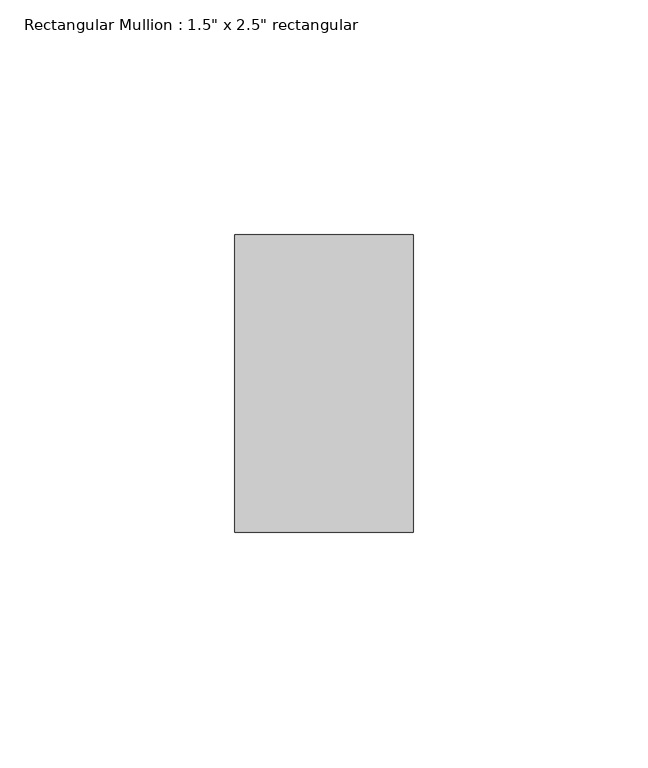
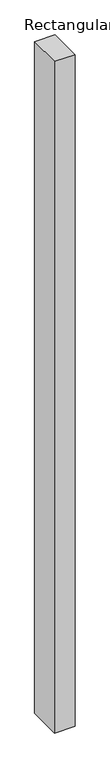
"""IFC4 building model written with IfcOpenShell, lengths in millimetres: member geometry."""

from ifc_helpers import new_model, si_unit, frame, origin, place, context, project, spatial, polyline, outline, extrude, source, transform, mapped, element, save


def member_030f819f(model_context):
    return source(origin(), model_context, "Body", "SweptSolid", [
        extrude(outline(polyline([(0.0, 31.75), (0.0, -31.75), (-38.1, -31.75), (-38.1, 31.75), (0.0, 31.75)])), frame((0.0, 0.0, -1315.2360761), z_axis=(0.0, 0.0, 1.0), x_axis=(1.0, 0.0, 0.0)), (0.0, 0.0, 1.0), 1315.2360761),
    ])


if __name__ == "__main__":
    model = new_model("IFC4")
    model_context = context("Model", 3, world=origin())
    ifc_project = project(units=[si_unit("LENGTHUNIT", "METRE", prefix="MILLI")], contexts=[model_context])
    site = spatial("IfcSite", under=ifc_project)
    building = spatial("IfcBuilding", under=site)
    placement = place(None, origin())
    member_shape = member_030f819f(model_context)
    element("IfcMember", 1, ObjectType="Rectangular Mullion : 1.5\" x 2.5\" rectangular", at=placement, inside=building, context=model_context, shape_type="MappedRepresentation", body=[
        mapped(member_shape, transform((0.0, 0.0, 0.0), x_axis=(1.0, 0.0, 0.0), y_axis=(0.0, 1.0, 0.0), z_axis=(0.0, 0.0, 1.0))),
    ])
    save(model, "model.ifc")

# Revit data of these elements
# Type "Rectangular Mullion : 1.5\" x 2.5\" rectangular"
#   built-in parameter 1007304 = 0.208333 (stored number, unit not read)
#   built-in parameter 1007301 = 0.0625 (stored number, unit not read)
#   built-in parameter 1007300 = 0.0625 (stored number, unit not read)
# Element 1 (IfcMember, "Rectangular Mullion : 1.5\" x 2.5\" rectangular")
#   Materials on its faces: "Damp-proofing"
# Materials
#   "Damp-proofing": class "Generic", colour RGB 127 127 127, transparency 0, Description = "Damp-proofing", Cost = 0
